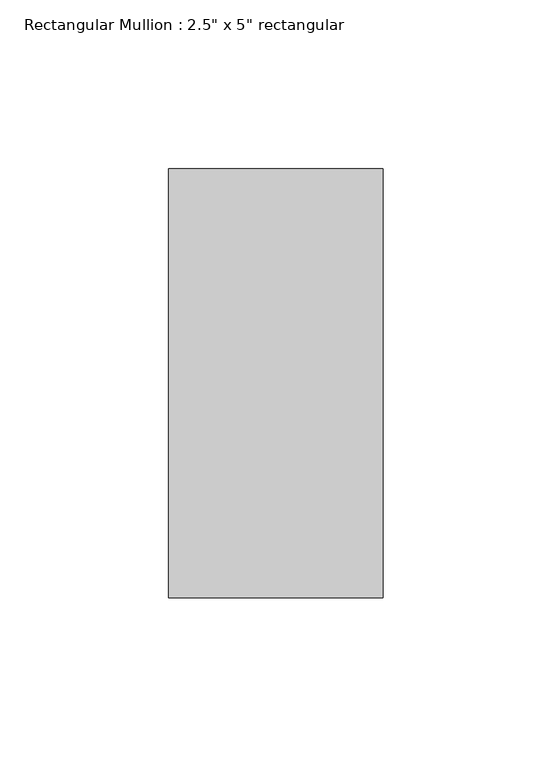
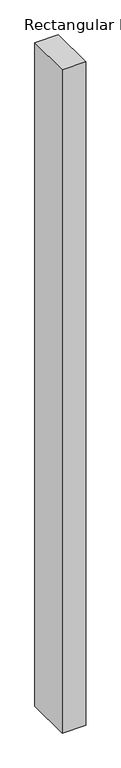
"""IFC4 building model written with IfcOpenShell, lengths in millimetres: member geometry."""

from ifc_helpers import new_model, si_unit, frame, origin, place, context, project, spatial, polyline, outline, extrude, source, transform, mapped, element, save


def member_52eebb51(model_context):
    return source(origin(), model_context, "Body", "SweptSolid", [
        extrude(outline(polyline([(0.0, 63.5), (0.0, -63.5), (-63.5, -63.5), (-63.5, 63.5), (0.0, 63.5)])), frame((0.0, 0.0, -1889.1776273), z_axis=(0.0, 0.0, 1.0), x_axis=(1.0, 0.0, 0.0)), (0.0, 0.0, 1.0), 1889.1776273),
    ])


if __name__ == "__main__":
    model = new_model("IFC4")
    model_context = context("Model", 3, world=origin())
    ifc_project = project(units=[si_unit("LENGTHUNIT", "METRE", prefix="MILLI")], contexts=[model_context])
    site = spatial("IfcSite", under=ifc_project)
    building = spatial("IfcBuilding", under=site)
    placement = place(None, origin())
    member_shape = member_52eebb51(model_context)
    element("IfcMember", 1, ObjectType="Rectangular Mullion : 2.5\" x 5\" rectangular", at=placement, inside=building, context=model_context, shape_type="MappedRepresentation", body=[
        mapped(member_shape, transform((0.0, 0.0, 0.0), x_axis=(1.0, 0.0, 0.0), y_axis=(0.0, 1.0, 0.0), z_axis=(0.0, 0.0, 1.0))),
    ])
    save(model, "model.ifc")

# Revit data of these elements
# Type "Rectangular Mullion : 2.5\" x 5\" rectangular"
#   built-in parameter 1007304 = 0.416667 (stored number, unit not read)
#   built-in parameter 1007301 = 0.104167 (stored number, unit not read)
#   built-in parameter 1007300 = 0.104167 (stored number, unit not read)
# Element 1 (IfcMember, "Rectangular Mullion : 2.5\" x 5\" rectangular")
#   Materials on its faces: "Aluminum"
# Materials
#   "Aluminum": class "Metal", colour RGB 247 247 247, transparency 0, Description = "Aluminum 6061", Cost = 0
